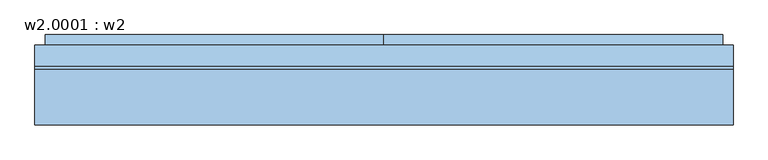
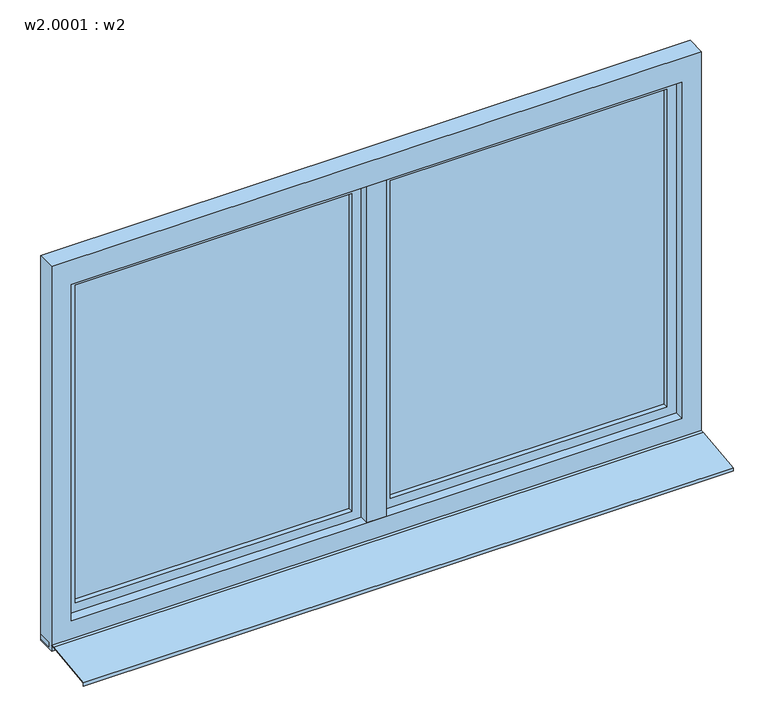
"""IFC4 building model written with IfcOpenShell, lengths in millimetres: window geometry, w2.0001 : w2."""

from ifc_helpers import new_model, si_unit, frame, origin, place, context, project, spatial, polyline, outline, extrude, faceted_brep, source, transform, mapped, element, save


def w2_0001_w2_6e690f8f(model_context):
    return source(origin(), model_context, "Body", "SolidModel", [
        extrude(outline(polyline([(66.4778457, 1020.0), (76.5, 1020.0), (76.5, 1018.0), (66.6759277, 1018.0), (-91.5, 998.3604634), (-91.5, 990.0), (-93.5, 990.0), (-93.5, 1000.0), (66.4778457, 1020.0)])), frame((-1005.0, 0.0, 0.0), z_axis=(1.0, 0.0, 0.0), x_axis=(0.0, 1.0, 0.0)), (0.0, 0.0, 1.0), 2010.0),
        extrude(outline(polyline([(-1005.0, 136.5), (1005.0, 136.5), (1005.0, 93.5), (-1005.0, 93.5), (-1005.0, 136.5)])), frame((0.0, 0.0, 1005.0), z_axis=(0.0, 0.0, 1.0), x_axis=(1.0, 0.0, 0.0)), (0.0, 0.0, 1.0), 15.0),
        extrude(outline(polyline([(60.0, 121.5), (60.0, 151.5), (915.0, 151.5), (915.0, 121.5), (60.0, 121.5)])), frame((0.0, 0.0, 1110.0), z_axis=(0.0, 0.0, 1.0), x_axis=(1.0, 0.0, 0.0)), (0.0, 0.0, 1.0), 1040.0),
        extrude(outline(polyline([(-915.0, 121.5), (-915.0, 151.5), (-60.0, 151.5), (-60.0, 121.5), (-915.0, 121.5)])), frame((0.0, 0.0, 1110.0), z_axis=(0.0, 0.0, 1.0), x_axis=(1.0, 0.0, 0.0)), (0.0, 0.0, 1.0), 1040.0),
        extrude(outline(polyline([(2260.0, -1005.0), (1000.0, -1005.0), (1000.0, 1005.0), (2260.0, 1005.0), (2260.0, -1005.0)]), holes=[polyline([(2180.0, -945.0), (2180.0, 945.0), (1080.0, 945.0), (1080.0, -945.0), (2180.0, -945.0)])]), frame((0.0, 76.5, 0.0), z_axis=(0.0, 1.0, 0.0), x_axis=(0.0, 0.0, 1.0)), (0.0, 0.0, 1.0), 60.0),
        extrude(outline(polyline([(30.0, 136.5), (30.0, 76.5), (-30.0, 76.5), (-30.0, 136.5), (30.0, 136.5)])), frame((0.0, 0.0, 1080.0), z_axis=(0.0, 0.0, 1.0), x_axis=(1.0, 0.0, 0.0)), (0.0, 0.0, 1.0), 1100.0),
        faceted_brep([(30.0, 136.5, 1080.0), (945.0, 136.5, 1080.0), (945.0, 106.5, 1080.0), (30.0, 106.5, 1080.0), (945.0, 136.5, 2180.0), (945.0, 106.5, 2180.0), (30.0, 106.5, 2180.0), (915.0, 106.5, 2150.0), (915.0, 106.5, 1110.0), (60.0, 106.5, 1110.0), (60.0, 106.5, 2150.0), (975.0, 136.5, 1050.0), (975.0, 136.5, 2210.0), (0.0, 136.5, 2210.0), (0.0, 136.5, 1050.0), (30.0, 136.5, 2180.0), (0.0, 166.5, 1050.0), (975.0, 166.5, 1050.0), (975.0, 166.5, 2210.0), (0.0, 166.5, 2210.0), (915.0, 166.5, 1110.0), (915.0, 166.5, 2150.0), (60.0, 166.5, 2150.0), (60.0, 166.5, 1110.0)], [[[0, 1, 2, 3]], [[1, 4, 5, 2]], [[2, 5, 6, 3], [7, 8, 9, 10]], [[11, 12, 13, 14], [4, 1, 0, 15]], [[16, 17, 11, 14]], [[17, 18, 12, 11]], [[18, 17, 16, 19], [20, 21, 22, 23]], [[9, 8, 20, 23]], [[8, 7, 21, 20]], [[15, 0, 3, 6]], [[19, 16, 14, 13]], [[10, 9, 23, 22]], [[4, 15, 6, 5]], [[18, 19, 13, 12]], [[7, 10, 22, 21]]]),
        faceted_brep([(-945.0, 136.5, 1080.0), (-30.0, 136.5, 1080.0), (-30.0, 106.5, 1080.0), (-945.0, 106.5, 1080.0), (-30.0, 136.5, 2180.0), (-30.0, 106.5, 2180.0), (-945.0, 106.5, 2180.0), (-60.0, 106.5, 2150.0), (-60.0, 106.5, 1110.0), (-915.0, 106.5, 1110.0), (-915.0, 106.5, 2150.0), (0.0, 136.5, 1050.0), (0.0, 136.5, 2210.0), (-975.0, 136.5, 2210.0), (-975.0, 136.5, 1050.0), (-945.0, 136.5, 2180.0), (-975.0, 166.5, 1050.0), (0.0, 166.5, 1050.0), (0.0, 166.5, 2210.0), (-975.0, 166.5, 2210.0), (-60.0, 166.5, 1110.0), (-60.0, 166.5, 2150.0), (-915.0, 166.5, 2150.0), (-915.0, 166.5, 1110.0)], [[[0, 1, 2, 3]], [[1, 4, 5, 2]], [[2, 5, 6, 3], [7, 8, 9, 10]], [[11, 12, 13, 14], [4, 1, 0, 15]], [[16, 17, 11, 14]], [[17, 18, 12, 11]], [[18, 17, 16, 19], [20, 21, 22, 23]], [[9, 8, 20, 23]], [[8, 7, 21, 20]], [[15, 0, 3, 6]], [[19, 16, 14, 13]], [[10, 9, 23, 22]], [[4, 15, 6, 5]], [[18, 19, 13, 12]], [[7, 10, 22, 21]]]),
    ])


if __name__ == "__main__":
    model = new_model("IFC4")
    model_context = context("Model", 3, world=origin())
    ifc_project = project(units=[si_unit("LENGTHUNIT", "METRE", prefix="MILLI")], contexts=[model_context])
    site = spatial("IfcSite", under=ifc_project)
    building = spatial("IfcBuilding", under=site)
    placement = place(None, origin())
    w2_0001_w2_shape = w2_0001_w2_6e690f8f(model_context)
    element("IfcWindow", 1, ObjectType="w2.0001 : w2", at=placement, inside=building, context=model_context, shape_type="MappedRepresentation", body=[
        mapped(w2_0001_w2_shape, transform((0.0, 0.0, 0.0), x_axis=(1.0, 0.0, 0.0), y_axis=(0.0, 1.0, 0.0), z_axis=(0.0, 0.0, 1.0))),
    ])
    save(model, "model.ifc")

# Revit data of these elements
# Type "w2.0001 : w2"
#   Type Mark = "19"
#   Operation = "DoublePanelVertical"
#   Keynote = "16.05.01"
#   Analytic Construction = "<None>"
#   Rough Width = 6' - 7.13386"
#   Rough Height = 4' - 1.6063"
#   Rahmentiefe = 0' - 2.3622"
#   Rahmenhöhe unten = 0' - 3.14961"
#   Rahmehöhe oben = 0' - 3.14961"
#   Rahmenbreite = 0' - 2.3622"
#   Height = 4' - 1.6063"
#   Flügeltiefe = 0' - 2.3622"
#   Flügelbreite = 0' - 2.3622"
#   Einbautiefe (von außen) [instance default] = 0' - 5.51181"
#   Width = 6' - 7.13386"
#   Kippflügel [instance default] = yes
#   Drehflügel im Grundriß darstellen [instance default] = no
#   Drehflügel [instance default] = yes
#   Define Thermal Properties by = 1
#   Rahmen [instance default] = none
#   Glas [instance default] = none
#   Flügel [instance default] = none
#   Fensterbank aussen [instance default] = none
#   Fensterbank innen [instance default] = none
#   Wall Closure = (empty or 0)
# Element 1 (IfcWindow, "w2.0001 : w2")
#   Materials on its faces: "Fenster - Kunststoff", "Fenster - Kunststoff weiss", "Glass", "Fenster - Holz"
# Materials
#   "Fenster - Kunststoff": colour RGB 249 249 249, transparency 0
#   "Fenster - Kunststoff weiss": colour RGB 249 249 249, transparency 0
#   "Glass": class "Glass", colour RGB 0 128 192, transparency 0.75, Description = "Soda Lime Glass", Cost = 0
#   "Fenster - Holz": colour RGB 216 135 75, transparency 0
